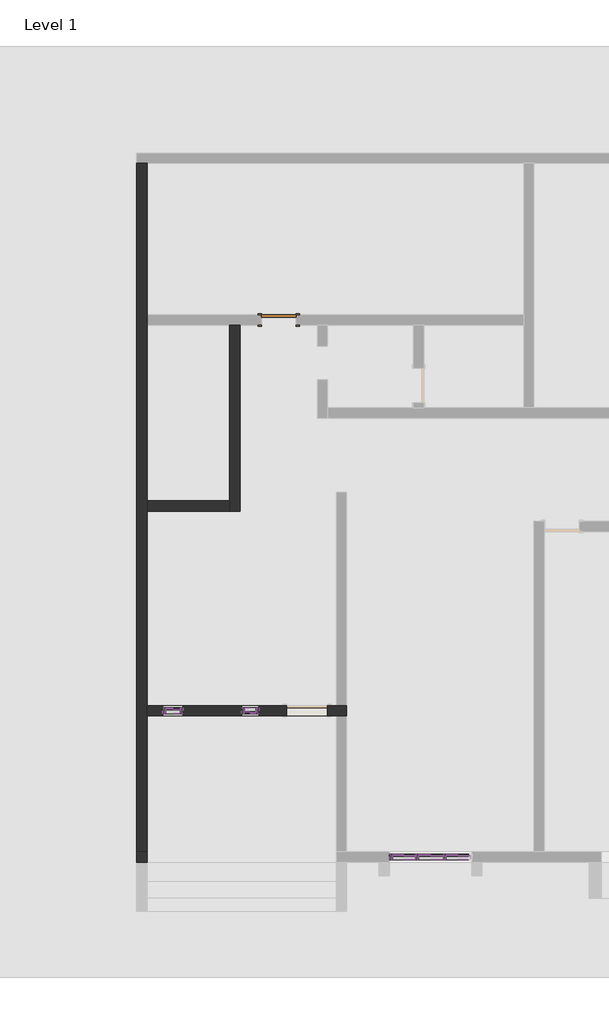
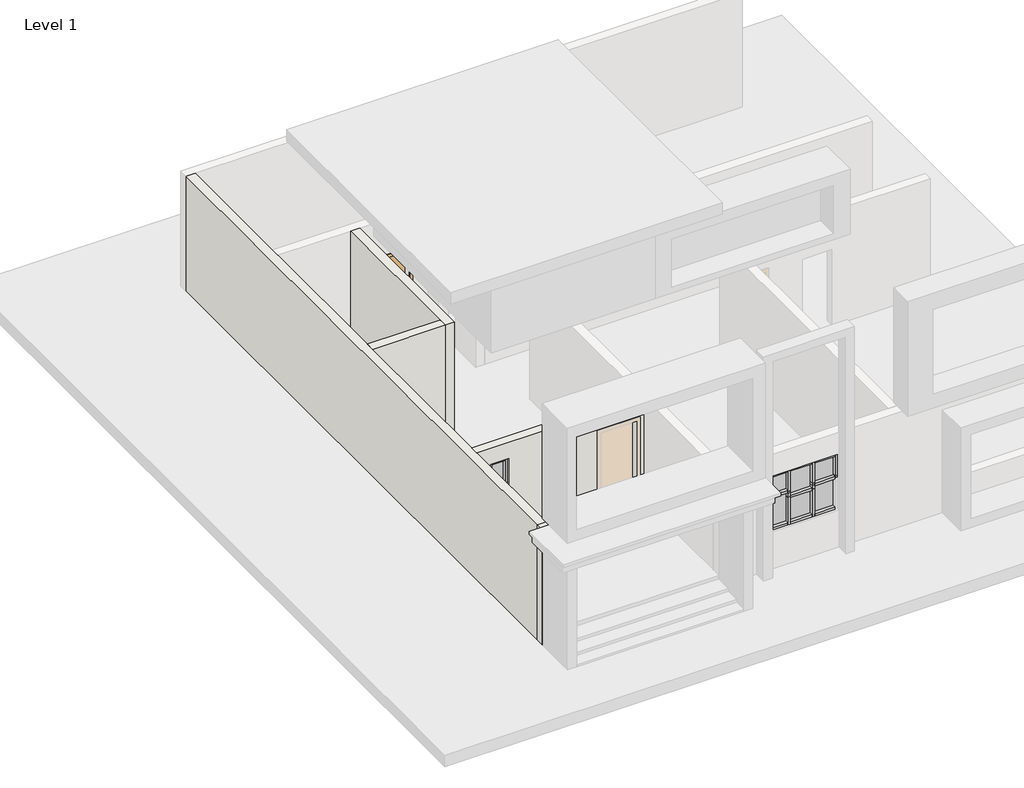
# One storey, part 1 of 2: 43 members, 12 plates, 5 walls, 1 door.
"""IFC4 building model written with IfcOpenShell, lengths in millimetres."""

from ifc_helpers import new_model, si_unit, origin, origin_with_axes, place, context, project, spatial, polyline, outline, extrude, faceted_brep, transform, mapped, element, save
from components import door_a1484949, member_21c47307, member_0c1408be, member_ff9f2d30, member_e97888c9, member_e59d5788, member_a44b2684, member_fb13da3b, member_67d1cd44, member_ea55af56, member_aaa03826, member_0b7646a3, member_06be906d, member_2c0166dc, member_cfc5edb3, member_a980948f, member_0a1a1ade, member_41360271, member_e61db9c9, system_panel_glazed_58f4fe82, system_panel_glazed_09b5f287, system_panel_glazed_e489fbe4, system_panel_glazed_b0e64c9e, system_panel_glazed_c28d2e47, system_panel_glazed_693ea391, system_panel_glazed_83ea90e8, system_panel_glazed_2d09ef22, system_panel_glazed_56d4eafa, system_panel_glazed_bf274a97

model = new_model("IFC4")

# Units and contexts
model_context = context("Model", 3, world=origin())
ifc_project = project(units=[si_unit("LENGTHUNIT", "METRE", prefix="MILLI")], contexts=[model_context])

# Site, building, storey
site = spatial("IfcSite", under=ifc_project)
building = spatial("IfcBuilding", under=site)
storey = spatial("IfcBuildingStorey", under=building, Name="Level 1", Elevation=0.0)

# Door
placement = place(None, origin())
door_shape = door_a1484949(model_context)
element("IfcDoor", 1, ObjectType="Single-Flush : 30\" x 80\"", at=placement, inside=storey, context=model_context, shape_type="MappedRepresentation", body=[
    mapped(door_shape, transform((-16045.8903308, -1353.8518738, 0.0), x_axis=(1.0, 0.0, 0.0), y_axis=(0.0, 1.0, 0.0), z_axis=(0.0, 0.0, 1.0))),
])

# Members
member_shape = member_21c47307(model_context)
element("IfcMember", 2, ObjectType="Rectangular Mullion : 2.5\" x 5\" rectangular", at=placement, inside=storey, context=model_context, shape_type="MappedRepresentation", body=[
    mapped(member_shape, transform((-18617.6403308, -10002.5518738, 1975.7481696), x_axis=(-1.0, 0.0, 0.0), y_axis=(0.0, -1.0, 0.0), z_axis=(0.0, 0.0, 1.0))),
])
element("IfcMember", 3, ObjectType="Rectangular Mullion : 2.5\" x 5\" rectangular", at=placement, inside=storey, context=model_context, shape_type="MappedRepresentation", body=[
    mapped(member_shape, transform((-18617.6403308, -10002.5518738, 1324.6334671), x_axis=(-1.0, 0.0, 0.0), y_axis=(0.0, -1.0, 0.0), z_axis=(0.0, 0.0, 1.0))),
])
element("IfcMember", 4, ObjectType="Rectangular Mullion : 2.5\" x 5\" rectangular", at=placement, inside=storey, context=model_context, shape_type="MappedRepresentation", body=[
    mapped(member_shape, transform((-18617.6403308, -10002.5518738, 2626.8628722), x_axis=(-1.0, 0.0, 0.0), y_axis=(0.0, -1.0, 0.0), z_axis=(0.0, 0.0, 1.0))),
])
member_2_shape = member_0c1408be(model_context)
element("IfcMember", 5, ObjectType="Rectangular Mullion : 2.5\" x 5\" rectangular", at=placement, inside=storey, context=model_context, shape_type="MappedRepresentation", body=[
    mapped(member_2_shape, transform((-18223.9403308, -10002.5518738, 1975.7481696), x_axis=(0.0, 0.0, 1.0), y_axis=(0.0, -1.0, 0.0), z_axis=(1.0, 0.0, 0.0))),
])
element("IfcMember", 6, ObjectType="Rectangular Mullion : 2.5\" x 5\" rectangular", at=placement, inside=storey, context=model_context, shape_type="MappedRepresentation", body=[
    mapped(member_2_shape, transform((-18223.9403308, -10002.5518738, 1324.6334671), x_axis=(0.0, 0.0, 1.0), y_axis=(0.0, -1.0, 0.0), z_axis=(1.0, 0.0, 0.0))),
])
member_3_shape = member_ff9f2d30(model_context)
element("IfcMember", 7, ObjectType="Rectangular Mullion : 2.5\" x 5\" rectangular", at=placement, inside=storey, context=model_context, shape_type="MappedRepresentation", body=[
    mapped(member_3_shape, transform((-18554.1403308, -10002.5518738, 673.5187645), x_axis=(0.0, 0.0, -1.0), y_axis=(0.0, -1.0, 0.0), z_axis=(-1.0, 0.0, 0.0))),
])
element("IfcMember", 8, ObjectType="Rectangular Mullion : 2.5\" x 5\" rectangular", at=placement, inside=storey, context=model_context, shape_type="MappedRepresentation", body=[
    mapped(member_3_shape, transform((-18223.9403308, -10002.5518738, 2626.8628722), x_axis=(0.0, 0.0, 1.0), y_axis=(0.0, -1.0, 0.0), z_axis=(1.0, 0.0, 0.0))),
])
element("IfcMember", 9, ObjectType="Rectangular Mullion : 2.5\" x 5\" rectangular", at=placement, inside=storey, context=model_context, shape_type="MappedRepresentation", body=[
    mapped(member_shape, transform((-18160.4403308, -10002.5518738, 1324.6334671), x_axis=(1.0, 0.0, 0.0), y_axis=(0.0, -1.0, 0.0), z_axis=(0.0, 0.0, -1.0))),
])
element("IfcMember", 10, ObjectType="Rectangular Mullion : 2.5\" x 5\" rectangular", at=placement, inside=storey, context=model_context, shape_type="MappedRepresentation", body=[
    mapped(member_shape, transform((-18160.4403308, -10002.5518738, 1975.7481696), x_axis=(1.0, 0.0, 0.0), y_axis=(0.0, -1.0, 0.0), z_axis=(0.0, 0.0, -1.0))),
])
element("IfcMember", 11, ObjectType="Rectangular Mullion : 2.5\" x 5\" rectangular", at=placement, inside=storey, context=model_context, shape_type="MappedRepresentation", body=[
    mapped(member_shape, transform((-18160.4403308, -10002.5518738, 673.5187645), x_axis=(1.0, 0.0, 0.0), y_axis=(0.0, -1.0, 0.0), z_axis=(0.0, 0.0, -1.0))),
])
member_4_shape = member_e97888c9(model_context)
element("IfcMember", 12, ObjectType="Rectangular Mullion : 2.5\" x 5\" rectangular", at=placement, inside=storey, context=model_context, shape_type="MappedRepresentation", body=[
    mapped(member_4_shape, transform((-16865.0403308, -10002.5518738, 1336.7072018), x_axis=(-1.0, 0.0, 0.0), y_axis=(0.0, 1.0, 0.0), z_axis=(0.0, 0.0, -1.0))),
])
element("IfcMember", 13, ObjectType="Rectangular Mullion : 2.5\" x 5\" rectangular", at=placement, inside=storey, context=model_context, shape_type="MappedRepresentation", body=[
    mapped(member_4_shape, transform((-16865.0403308, -10002.5518738, 644.2714463), x_axis=(-1.0, 0.0, 0.0), y_axis=(0.0, 1.0, 0.0), z_axis=(0.0, 0.0, -1.0))),
])
element("IfcMember", 14, ObjectType="Rectangular Mullion : 2.5\" x 5\" rectangular", at=placement, inside=storey, context=model_context, shape_type="MappedRepresentation", body=[
    mapped(member_4_shape, transform((-16865.0403308, -10002.5518738, 2029.1429573), x_axis=(-1.0, 0.0, 0.0), y_axis=(0.0, 1.0, 0.0), z_axis=(0.0, 0.0, -1.0))),
])
member_5_shape = member_e59d5788(model_context)
element("IfcMember", 15, ObjectType="Rectangular Mullion : 2.5\" x 5\" rectangular", at=placement, inside=storey, context=model_context, shape_type="MappedRepresentation", body=[
    mapped(member_5_shape, transform((-16801.5403308, -10002.5518738, 1336.7072018), x_axis=(0.0, 0.0, 1.0), y_axis=(0.0, 1.0, 0.0), z_axis=(-1.0, 0.0, 0.0))),
])
element("IfcMember", 16, ObjectType="Rectangular Mullion : 2.5\" x 5\" rectangular", at=placement, inside=storey, context=model_context, shape_type="MappedRepresentation", body=[
    mapped(member_5_shape, transform((-16801.5403308, -10002.5518738, 2029.1429573), x_axis=(0.0, 0.0, 1.0), y_axis=(0.0, 1.0, 0.0), z_axis=(-1.0, 0.0, 0.0))),
])
member_6_shape = member_a44b2684(model_context)
element("IfcMember", 17, ObjectType="Rectangular Mullion : 2.5\" x 5\" rectangular", at=placement, inside=storey, context=model_context, shape_type="MappedRepresentation", body=[
    mapped(member_6_shape, transform((-16547.5403308, -10002.5518738, 644.2714463), x_axis=(0.0, 0.0, -1.0), y_axis=(0.0, 1.0, 0.0), z_axis=(1.0, 0.0, 0.0))),
])
element("IfcMember", 18, ObjectType="Rectangular Mullion : 2.5\" x 5\" rectangular", at=placement, inside=storey, context=model_context, shape_type="MappedRepresentation", body=[
    mapped(member_6_shape, transform((-16801.5403308, -10002.5518738, 2721.5787129), x_axis=(0.0, 0.0, 1.0), y_axis=(0.0, 1.0, 0.0), z_axis=(-1.0, 0.0, 0.0))),
])
element("IfcMember", 19, ObjectType="Rectangular Mullion : 2.5\" x 5\" rectangular", at=placement, inside=storey, context=model_context, shape_type="MappedRepresentation", body=[
    mapped(member_4_shape, transform((-16484.0403308, -10002.5518738, 1336.7072018), x_axis=(1.0, 0.0, 0.0), y_axis=(0.0, 1.0, 0.0), z_axis=(0.0, 0.0, 1.0))),
])
element("IfcMember", 20, ObjectType="Rectangular Mullion : 2.5\" x 5\" rectangular", at=placement, inside=storey, context=model_context, shape_type="MappedRepresentation", body=[
    mapped(member_4_shape, transform((-16484.0403308, -10002.5518738, 2029.1429573), x_axis=(1.0, 0.0, 0.0), y_axis=(0.0, 1.0, 0.0), z_axis=(0.0, 0.0, 1.0))),
])
element("IfcMember", 21, ObjectType="Rectangular Mullion : 2.5\" x 5\" rectangular", at=placement, inside=storey, context=model_context, shape_type="MappedRepresentation", body=[
    mapped(member_4_shape, transform((-16484.0403308, -10002.5518738, 2721.5787129), x_axis=(1.0, 0.0, 0.0), y_axis=(0.0, 1.0, 0.0), z_axis=(0.0, 0.0, 1.0))),
])
member_7_shape = member_fb13da3b(model_context)
element("IfcMember", 22, ObjectType="Rectangular Mullion : 2.5\" x 5\" rectangular", at=placement, inside=storey, context=model_context, shape_type="MappedRepresentation", body=[
    mapped(member_7_shape, transform((-13588.4403308, -13241.0518738, 1825.4543679), x_axis=(-1.0, 0.0, 0.0), y_axis=(0.0, -1.0, 0.0), z_axis=(0.0, 0.0, 1.0))),
])
member_8_shape = member_67d1cd44(model_context)
element("IfcMember", 23, ObjectType="Rectangular Mullion : 2.5\" x 5\" rectangular", at=placement, inside=storey, context=model_context, shape_type="MappedRepresentation", body=[
    mapped(member_8_shape, transform((-13588.4403308, -13241.0518738, 1876.2543679), x_axis=(-1.0, 0.0, 0.0), y_axis=(0.0, -1.0, 0.0), z_axis=(0.0, 0.0, 1.0))),
])
member_9_shape = member_ea55af56(model_context)
element("IfcMember", 24, ObjectType="Rectangular Mullion : 2.5\" x 5\" rectangular", at=placement, inside=storey, context=model_context, shape_type="MappedRepresentation", body=[
    mapped(member_9_shape, transform((-13588.4403308, -13241.0518738, 2460.1511243), x_axis=(-1.0, 0.0, 0.0), y_axis=(0.0, -1.0, 0.0), z_axis=(0.0, 0.0, 1.0))),
])
member_10_shape = member_aaa03826(model_context)
element("IfcMember", 25, ObjectType="Rectangular Mullion : 2.5\" x 5\" rectangular", at=placement, inside=storey, context=model_context, shape_type="MappedRepresentation", body=[
    mapped(member_10_shape, transform((-13010.5903308, -13241.0518738, 1876.2543679), x_axis=(0.0, 0.0, 1.0), y_axis=(0.0, -1.0, 0.0), z_axis=(1.0, 0.0, 0.0))),
])
element("IfcMember", 26, ObjectType="Rectangular Mullion : 2.5\" x 5\" rectangular", at=placement, inside=storey, context=model_context, shape_type="MappedRepresentation", body=[
    mapped(member_10_shape, transform((-11823.1403308, -13241.0518738, 1825.4543679), x_axis=(0.0, 0.0, 1.0), y_axis=(0.0, -1.0, 0.0), z_axis=(1.0, 0.0, 0.0))),
])
member_11_shape = member_0b7646a3(model_context)
element("IfcMember", 27, ObjectType="Rectangular Mullion : 2.5\" x 5\" rectangular", at=placement, inside=storey, context=model_context, shape_type="MappedRepresentation", body=[
    mapped(member_11_shape, transform((-13010.5903308, -13241.0518738, 2460.1511243), x_axis=(0.0, 0.0, 1.0), y_axis=(0.0, -1.0, 0.0), z_axis=(1.0, 0.0, 0.0))),
])
element("IfcMember", 28, ObjectType="Rectangular Mullion : 2.5\" x 5\" rectangular", at=placement, inside=storey, context=model_context, shape_type="MappedRepresentation", body=[
    mapped(member_11_shape, transform((-11823.1403308, -13241.0518738, 2460.1511243), x_axis=(0.0, 0.0, 1.0), y_axis=(0.0, -1.0, 0.0), z_axis=(1.0, 0.0, 0.0))),
])
member_12_shape = member_06be906d(model_context)
element("IfcMember", 29, ObjectType="Rectangular Mullion : 2.5\" x 5\" rectangular", at=placement, inside=storey, context=model_context, shape_type="MappedRepresentation", body=[
    mapped(member_12_shape, transform((-12978.8403308, -13241.0518738, 1825.4543679), x_axis=(1.0, 0.0, 0.0), y_axis=(0.0, -1.0, 0.0), z_axis=(0.0, 0.0, -1.0))),
])
member_13_shape = member_2c0166dc(model_context)
element("IfcMember", 30, ObjectType="Rectangular Mullion : 2.5\" x 5\" rectangular", at=placement, inside=storey, context=model_context, shape_type="MappedRepresentation", body=[
    mapped(member_13_shape, transform((-12978.8403308, -13241.0518738, 1876.2543679), x_axis=(1.0, 0.0, 0.0), y_axis=(0.0, -1.0, 0.0), z_axis=(0.0, 0.0, -1.0))),
])
member_14_shape = member_cfc5edb3(model_context)
element("IfcMember", 31, ObjectType="Rectangular Mullion : 2.5\" x 5\" rectangular", at=placement, inside=storey, context=model_context, shape_type="MappedRepresentation", body=[
    mapped(member_14_shape, transform((-12978.8403308, -13241.0518738, 1723.8543679), x_axis=(1.0, 0.0, 0.0), y_axis=(0.0, -1.0, 0.0), z_axis=(0.0, 0.0, -1.0))),
])
member_15_shape = member_a980948f(model_context)
element("IfcMember", 32, ObjectType="Rectangular Mullion : 2.5\" x 5\" rectangular", at=placement, inside=storey, context=model_context, shape_type="MappedRepresentation", body=[
    mapped(member_15_shape, transform((-12400.9903308, -13241.0518738, 2460.1511243), x_axis=(0.0, 0.0, 1.0), y_axis=(0.0, -1.0, 0.0), z_axis=(1.0, 0.0, 0.0))),
])
member_16_shape = member_0a1a1ade(model_context)
element("IfcMember", 33, ObjectType="Rectangular Mullion : 2.5\" x 5\" rectangular", at=placement, inside=storey, context=model_context, shape_type="MappedRepresentation", body=[
    mapped(member_16_shape, transform((-12400.9903308, -13241.0518738, 1723.8543679), x_axis=(0.0, 0.0, 1.0), y_axis=(0.0, -1.0, 0.0), z_axis=(1.0, 0.0, 0.0))),
])
element("IfcMember", 34, ObjectType="Rectangular Mullion : 2.5\" x 5\" rectangular", at=placement, inside=storey, context=model_context, shape_type="MappedRepresentation", body=[
    mapped(member_13_shape, transform((-12369.2403308, -13241.0518738, 1876.2543679), x_axis=(1.0, 0.0, 0.0), y_axis=(0.0, -1.0, 0.0), z_axis=(0.0, 0.0, -1.0))),
])
element("IfcMember", 35, ObjectType="Rectangular Mullion : 2.5\" x 5\" rectangular", at=placement, inside=storey, context=model_context, shape_type="MappedRepresentation", body=[
    mapped(member_12_shape, transform((-12369.2403308, -13241.0518738, 1825.4543679), x_axis=(1.0, 0.0, 0.0), y_axis=(0.0, -1.0, 0.0), z_axis=(0.0, 0.0, -1.0))),
])
element("IfcMember", 36, ObjectType="Rectangular Mullion : 2.5\" x 5\" rectangular", at=placement, inside=storey, context=model_context, shape_type="MappedRepresentation", body=[
    mapped(member_14_shape, transform((-12369.2403308, -13241.0518738, 1723.8543679), x_axis=(1.0, 0.0, 0.0), y_axis=(0.0, -1.0, 0.0), z_axis=(0.0, 0.0, -1.0))),
])
element("IfcMember", 37, ObjectType="Rectangular Mullion : 2.5\" x 5\" rectangular", at=placement, inside=storey, context=model_context, shape_type="MappedRepresentation", body=[
    mapped(member_8_shape, transform((-11759.6403308, -13241.0518738, 1825.4543679), x_axis=(1.0, 0.0, 0.0), y_axis=(0.0, -1.0, 0.0), z_axis=(0.0, 0.0, -1.0))),
])
element("IfcMember", 38, ObjectType="Rectangular Mullion : 2.5\" x 5\" rectangular", at=placement, inside=storey, context=model_context, shape_type="MappedRepresentation", body=[
    mapped(member_9_shape, transform((-11759.6403308, -13241.0518738, 1876.2543679), x_axis=(1.0, 0.0, 0.0), y_axis=(0.0, -1.0, 0.0), z_axis=(0.0, 0.0, -1.0))),
])
member_17_shape = member_41360271(model_context)
element("IfcMember", 39, ObjectType="Rectangular Mullion : 2.5\" x 5\" rectangular", at=placement, inside=storey, context=model_context, shape_type="MappedRepresentation", body=[
    mapped(member_17_shape, transform((-12978.8403308, -13241.0518738, 987.5576115), x_axis=(1.0, 0.0, 0.0), y_axis=(0.0, -1.0, 0.0), z_axis=(0.0, 0.0, -1.0))),
])
element("IfcMember", 40, ObjectType="Rectangular Mullion : 2.5\" x 5\" rectangular", at=placement, inside=storey, context=model_context, shape_type="MappedRepresentation", body=[
    mapped(member_17_shape, transform((-12369.2403308, -13241.0518738, 987.5576115), x_axis=(1.0, 0.0, 0.0), y_axis=(0.0, -1.0, 0.0), z_axis=(0.0, 0.0, -1.0))),
])
element("IfcMember", 41, ObjectType="Rectangular Mullion : 2.5\" x 5\" rectangular", at=placement, inside=storey, context=model_context, shape_type="MappedRepresentation", body=[
    mapped(member_11_shape, transform((-12337.4903308, -13241.0518738, 987.5576115), x_axis=(0.0, 0.0, -1.0), y_axis=(0.0, -1.0, 0.0), z_axis=(-1.0, 0.0, 0.0))),
])
element("IfcMember", 42, ObjectType="Rectangular Mullion : 2.5\" x 5\" rectangular", at=placement, inside=storey, context=model_context, shape_type="MappedRepresentation", body=[
    mapped(member_11_shape, transform((-13524.9403308, -13241.0518738, 987.5576115), x_axis=(0.0, 0.0, -1.0), y_axis=(0.0, -1.0, 0.0), z_axis=(-1.0, 0.0, 0.0))),
])
element("IfcMember", 43, ObjectType="Rectangular Mullion : 2.5\" x 5\" rectangular", at=placement, inside=storey, context=model_context, shape_type="MappedRepresentation", body=[
    mapped(member_15_shape, transform((-12947.0903308, -13241.0518738, 987.5576115), x_axis=(0.0, 0.0, -1.0), y_axis=(0.0, -1.0, 0.0), z_axis=(-1.0, 0.0, 0.0))),
])
member_18_shape = member_e61db9c9(model_context)
element("IfcMember", 44, ObjectType="Rectangular Mullion : 2.5\" x 5\" rectangular", at=placement, inside=storey, context=model_context, shape_type="MappedRepresentation", body=[
    mapped(member_18_shape, transform((-13588.4403308, -13241.0518738, 1723.8543679), x_axis=(-1.0, 0.0, 0.0), y_axis=(0.0, -1.0, 0.0), z_axis=(0.0, 0.0, 1.0))),
])

# Plates
system_panel_glazed_shape = system_panel_glazed_58f4fe82(model_context)
element("IfcPlate", 45, ObjectType="System Panel : Glazed", at=placement, inside=storey, context=model_context, shape_type="MappedRepresentation", body=[
    mapped(system_panel_glazed_shape, transform((-18389.0403308, -10002.5518738, 737.0187645), x_axis=(1.0, 0.0, 0.0), y_axis=(0.0, 1.0, 0.0), z_axis=(0.0, 0.0, 1.0))),
])
element("IfcPlate", 46, ObjectType="System Panel : Glazed", at=placement, inside=storey, context=model_context, shape_type="MappedRepresentation", body=[
    mapped(system_panel_glazed_shape, transform((-18389.0403308, -10002.5518738, 2007.4981696), x_axis=(1.0, 0.0, 0.0), y_axis=(0.0, 1.0, 0.0), z_axis=(0.0, 0.0, 1.0))),
])
system_panel_glazed_2_shape = system_panel_glazed_09b5f287(model_context)
element("IfcPlate", 47, ObjectType="System Panel : Glazed", at=placement, inside=storey, context=model_context, shape_type="MappedRepresentation", body=[
    mapped(system_panel_glazed_2_shape, transform((-18389.0403308, -10002.5518738, 1356.3834671), x_axis=(1.0, 0.0, 0.0), y_axis=(0.0, 1.0, 0.0), z_axis=(0.0, 0.0, 1.0))),
])
system_panel_glazed_3_shape = system_panel_glazed_e489fbe4(model_context)
element("IfcPlate", 48, ObjectType="System Panel : Glazed", at=placement, inside=storey, context=model_context, shape_type="MappedRepresentation", body=[
    mapped(system_panel_glazed_3_shape, transform((-16674.5403308, -10002.5518738, 707.7714463), x_axis=(-1.0, 0.0, 0.0), y_axis=(0.0, -1.0, 0.0), z_axis=(0.0, 0.0, 1.0))),
])
element("IfcPlate", 49, ObjectType="System Panel : Glazed", at=placement, inside=storey, context=model_context, shape_type="MappedRepresentation", body=[
    mapped(system_panel_glazed_3_shape, transform((-16674.5403308, -10002.5518738, 2060.8929573), x_axis=(-1.0, 0.0, 0.0), y_axis=(0.0, -1.0, 0.0), z_axis=(0.0, 0.0, 1.0))),
])
system_panel_glazed_4_shape = system_panel_glazed_b0e64c9e(model_context)
element("IfcPlate", 50, ObjectType="System Panel : Glazed", at=placement, inside=storey, context=model_context, shape_type="MappedRepresentation", body=[
    mapped(system_panel_glazed_4_shape, transform((-16674.5403308, -10002.5518738, 1368.4572018), x_axis=(-1.0, 0.0, 0.0), y_axis=(0.0, -1.0, 0.0), z_axis=(0.0, 0.0, 1.0))),
])
system_panel_glazed_5_shape = system_panel_glazed_c28d2e47(model_context)
element("IfcPlate", 51, ObjectType="System Panel : Glazed", at=placement, inside=storey, context=model_context, shape_type="MappedRepresentation", body=[
    mapped(system_panel_glazed_5_shape, transform((-13267.7653308, -13241.0518738, 1908.0043679), x_axis=(1.0, 0.0, 0.0), y_axis=(0.0, 1.0, 0.0), z_axis=(0.0, 0.0, 1.0))),
])
system_panel_glazed_6_shape = system_panel_glazed_693ea391(model_context)
element("IfcPlate", 52, ObjectType="System Panel : Glazed", at=placement, inside=storey, context=model_context, shape_type="MappedRepresentation", body=[
    mapped(system_panel_glazed_6_shape, transform((-12674.0403308, -13241.0518738, 1755.6043679), x_axis=(1.0, 0.0, 0.0), y_axis=(0.0, 1.0, 0.0), z_axis=(0.0, 0.0, 1.0))),
])
system_panel_glazed_7_shape = system_panel_glazed_83ea90e8(model_context)
element("IfcPlate", 53, ObjectType="System Panel : Glazed", at=placement, inside=storey, context=model_context, shape_type="MappedRepresentation", body=[
    mapped(system_panel_glazed_7_shape, transform((-12080.3153308, -13241.0518738, 1857.2043679), x_axis=(1.0, 0.0, 0.0), y_axis=(0.0, 1.0, 0.0), z_axis=(0.0, 0.0, 1.0))),
])
system_panel_glazed_8_shape = system_panel_glazed_2d09ef22(model_context)
element("IfcPlate", 54, ObjectType="System Panel : Glazed", at=placement, inside=storey, context=model_context, shape_type="MappedRepresentation", body=[
    mapped(system_panel_glazed_8_shape, transform((-13267.7653308, -13241.0518738, 1051.0576115), x_axis=(1.0, 0.0, 0.0), y_axis=(0.0, 1.0, 0.0), z_axis=(0.0, 0.0, 1.0))),
])
system_panel_glazed_9_shape = system_panel_glazed_56d4eafa(model_context)
element("IfcPlate", 55, ObjectType="System Panel : Glazed", at=placement, inside=storey, context=model_context, shape_type="MappedRepresentation", body=[
    mapped(system_panel_glazed_9_shape, transform((-12674.0403308, -13241.0518738, 1051.0576115), x_axis=(1.0, 0.0, 0.0), y_axis=(0.0, 1.0, 0.0), z_axis=(0.0, 0.0, 1.0))),
])
system_panel_glazed_10_shape = system_panel_glazed_bf274a97(model_context)
element("IfcPlate", 56, ObjectType="System Panel : Glazed", at=placement, inside=storey, context=model_context, shape_type="MappedRepresentation", body=[
    mapped(system_panel_glazed_10_shape, transform((-12080.3153308, -13241.0518738, 1051.0576115), x_axis=(1.0, 0.0, 0.0), y_axis=(0.0, 1.0, 0.0), z_axis=(0.0, 0.0, 1.0))),
])

# Walls
element("IfcWall", 57, ObjectType="9\"", at=placement, inside=storey, context=model_context, shape_type="SweptSolid", body=[
    extrude(outline(polyline([(-18960.5403308, -13355.3518738), (-19189.1403308, -13355.3518738), (-19189.1403308, -13126.7518738), (-18960.5403308, -13126.7518738), (-18960.5403308, -13355.3518738)])), origin_with_axes(), (0.0, 0.0, 1.0), 3048.0),
])
element("IfcWall", 58, ObjectType="9\"", at=placement, inside=storey, context=model_context, shape_type="Brep", body=[
    faceted_brep([(-19189.1403308, 2113.2481262, 0.0), (-19189.1403308, -13126.7518738, 0.0), (-19189.1403308, -13126.7518738, 3048.0), (-19189.1403308, 2113.2481262, 3048.0), (-18960.5403308, 2113.2481262, 0.0), (-18960.5403308, 2113.2481262, 3048.0), (-18960.5403308, -1239.5518738, 3048.0), (-18960.5403308, -1468.1518738, 3048.0), (-18960.5403308, -5354.3518738, 3048.0), (-18960.5403308, -5582.9518738, 3048.0), (-18960.5403308, -9888.2518738, 3048.0), (-18960.5403308, -10116.8518738, 3048.0), (-18960.5403308, -13126.7518738, 3048.0), (-18960.5403308, -13126.7518738, 0.0), (-18960.5403308, -10116.8518738, 0.0), (-18960.5403308, -9888.2518738, 0.0), (-18960.5403308, -5582.9518738, 0.0), (-18960.5403308, -5354.3518738, 0.0), (-18960.5403308, -1468.1518738, 0.0), (-18960.5403308, -1239.5518738, 0.0)], [[[0, 1, 2, 3]], [[4, 5, 6, 7, 8, 9, 10, 11, 12, 13, 14, 15, 16, 17, 18, 19]], [[1, 0, 4, 19, 18, 17, 16, 15, 14, 13]], [[3, 2, 12, 11, 10, 9, 8, 7, 6, 5]], [[0, 3, 5, 4]], [[2, 1, 13, 12]]]),
])
element("IfcWall", 59, ObjectType="9\"", at=placement, inside=storey, context=model_context, shape_type="Brep", body=[
    faceted_brep([(-18960.5403308, -10116.8518738, 0.0), (-14769.5403308, -10116.8518738, 0.0), (-14540.9403308, -10116.8518738, 0.0), (-14540.9403308, -10116.8518738, 3048.0), (-14769.5403308, -10116.8518738, 3048.0), (-18960.5403308, -10116.8518738, 3048.0), (-14960.0403308, -10116.8518738, 381.0), (-15874.4403308, -10116.8518738, 381.0), (-15874.4403308, -10116.8518738, 2514.6), (-14960.0403308, -10116.8518738, 2514.6), (-18617.6403308, -10116.8518738, 673.5187645), (-18617.6403308, -10116.8518738, 2626.8628722), (-18160.4403308, -10116.8518738, 2626.8628722), (-18160.4403308, -10116.8518738, 673.5187645), (-16484.0403308, -10116.8518738, 2721.5787129), (-16484.0403308, -10116.8518738, 644.2714463), (-16865.0403308, -10116.8518738, 644.2714463), (-16865.0403308, -10116.8518738, 2721.5787129), (-14540.9403308, -9888.2518738, 0.0), (-14769.5403308, -9888.2518738, 0.0), (-18960.5403308, -9888.2518738, 0.0), (-18960.5403308, -9888.2518738, 3048.0), (-14769.5403308, -9888.2518738, 3048.0), (-14540.9403308, -9888.2518738, 3048.0), (-15874.4403308, -9888.2518738, 381.0), (-14960.0403308, -9888.2518738, 381.0), (-14960.0403308, -9888.2518738, 2514.6), (-15874.4403308, -9888.2518738, 2514.6), (-18617.6403308, -9888.2518738, 2626.8628722), (-18617.6403308, -9888.2518738, 673.5187645), (-18160.4403308, -9888.2518738, 673.5187645), (-18160.4403308, -9888.2518738, 2626.8628722), (-16484.0403308, -9888.2518738, 644.2714463), (-16484.0403308, -9888.2518738, 2721.5787129), (-16865.0403308, -9888.2518738, 2721.5787129), (-16865.0403308, -9888.2518738, 644.2714463)], [[[0, 1, 2, 3, 4, 5], [6, 7, 8, 9], [10, 11, 12, 13], [14, 15, 16, 17]], [[18, 19, 20, 21, 22, 23], [24, 25, 26, 27], [28, 29, 30, 31], [32, 33, 34, 35]], [[2, 1, 0, 20, 19, 18]], [[5, 4, 3, 23, 22, 21]], [[0, 5, 21, 20]], [[3, 2, 18, 23]], [[25, 24, 7, 6]], [[26, 25, 6, 9]], [[27, 26, 9, 8]], [[24, 27, 8, 7]], [[10, 29, 28, 11]], [[11, 28, 31, 12]], [[12, 31, 30, 13]], [[29, 10, 13, 30]], [[32, 15, 14, 33]], [[33, 14, 17, 34]], [[16, 35, 34, 17]], [[15, 32, 35, 16]]]),
])
element("IfcWall", 60, ObjectType="9\"", at=placement, inside=storey, context=model_context, shape_type="Brep", body=[
    faceted_brep([(-17131.7403308, -1468.1518738, 0.0), (-17131.7403308, -5354.3518738, 0.0), (-17131.7403308, -5582.9518738, 0.0), (-17131.7403308, -5582.9518738, 3048.0), (-17131.7403308, -5354.3518738, 3048.0), (-17131.7403308, -1468.1518738, 3048.0), (-16903.1403308, -1468.1518738, 0.0), (-16903.1403308, -1468.1518738, 3048.0), (-16903.1403308, -5582.9518738, 3048.0), (-16903.1403308, -5582.9518738, 0.0)], [[[0, 1, 2, 3, 4, 5]], [[6, 7, 8, 9]], [[2, 1, 0, 6, 9]], [[5, 4, 3, 8, 7]], [[0, 5, 7, 6]], [[3, 2, 9, 8]]]),
])
element("IfcWall", 61, ObjectType="9\"", at=placement, inside=storey, context=model_context, shape_type="SweptSolid", body=[
    extrude(outline(polyline([(-18960.5403308, -5354.3518738), (-17131.7403308, -5354.3518738), (-17131.7403308, -5582.9518738), (-18960.5403308, -5582.9518738), (-18960.5403308, -5354.3518738)])), origin_with_axes(), (0.0, 0.0, 1.0), 3048.0),
])

save(model, "model.ifc")

# Revit data of these elements
# Type "Single-Flush : 30\" x 80\""
#   Type Mark = "5"
#   Construction Type Id = "MDOOR"
#   Assembly Code = "C1020"
#   Analytic Construction = "Metal"
#   Thickness = 0' - 2"
#   Heat Transfer Coefficient (U) = 0.651978 BTU/(h·ft²·°F)
#   Height = 6' - 8"
#   Trim Projection Ext = 0' - 1"
#   Trim Projection Int = 0' - 1"
#   Trim Width = 0' - 3"
#   Width = 2' - 6"
#   Define Thermal Properties by = 1
#   Define Thermal Properties by = 1
#   Door Material = Door - Panel
#   Frame Material = Door - Frame
#   Visual Light Transmittance = 0
#   Solar Heat Gain Coefficient = 0
#   Function = (empty or 0)
#   Wall Closure = (empty or 0)
# Type "Rectangular Mullion : 2.5\" x 5\" rectangular"
#   built-in parameter 1007304 = 0.416667 (stored number, unit not read)
#   built-in parameter 1007301 = 0.104167 (stored number, unit not read)
#   built-in parameter 1007300 = 0.104167 (stored number, unit not read)
# Type "System Panel : Glazed"
#   Construction Type Id = "GSP4R"
#   Analytic Construction = "1/8 in Pilkington single glazing"
#   Visual Light Transmittance = 0.9
#   Solar Heat Gain Coefficient = 0.86
#   Heat Transfer Coefficient (U) = 1.18115 BTU/(h·ft²·°F)
#   Define Thermal Properties by = 1
# Type "9\""
#   Assembly Code = "B2010"
#   Layers, outside or top first: 0' - 9" no material (function 1)
# Element 1 (IfcDoor, "Single-Flush : 30\" x 80\"")
#   Phase Created = New Construction
#   Materials on its faces: "Door - Frame", "Door - Panel"
# Elements 2, 3, 4, 5, 6, 7, 8, 9, 10, 11, 12, 13, 14, 15, 16, 17, 18, 19, 20, 21, 22, 23, 24, 25, 26, 27, 28, 29, 30, 31, 32, 33, 34, 35, 36, 37, 38, 39, 40, 41, 42, 43, 44 (IfcMember, "Rectangular Mullion : 2.5\" x 5\" rectangular")
#   Phase Created = New Construction
#   Materials on its faces: "Aluminum"
# Elements 45, 46, 47, 48, 49, 50, 51, 52, 53, 54, 55, 56 (IfcPlate, "System Panel : Glazed")
#   Phase Created = New Construction
#   Materials on its faces: "Glass"
# Elements 57, 58, 59, 60, 61 (IfcWall, "9\"")
#   Top Offset = 0' - 0"
#   Base Offset = 0' - 0"
#   Unconnected Height = 10' - 0"
#   wall height = 10' - 0"
#   Phase Created = New Construction
#   Base Constraint = Level 1
#   Materials on its faces: "Default Wall"
# Materials
#   "Door - Panel": class "Wood", colour RGB 210 159 95, transparency 0, Cost = 0
#   "Door - Frame": colour RGB 118 70 51, transparency 0, Cost = 0
#   "Aluminum": class "Metal", colour RGB 247 247 247, transparency 0, Description = "Aluminum 6061", Cost = 0
#   "Glass": class "Glass", colour RGB 0 128 192, transparency 0.75, Description = "Soda Lime Glass", Cost = 0
#   "Default Wall": colour RGB 128 128 128, transparency 0, Cost = 0
